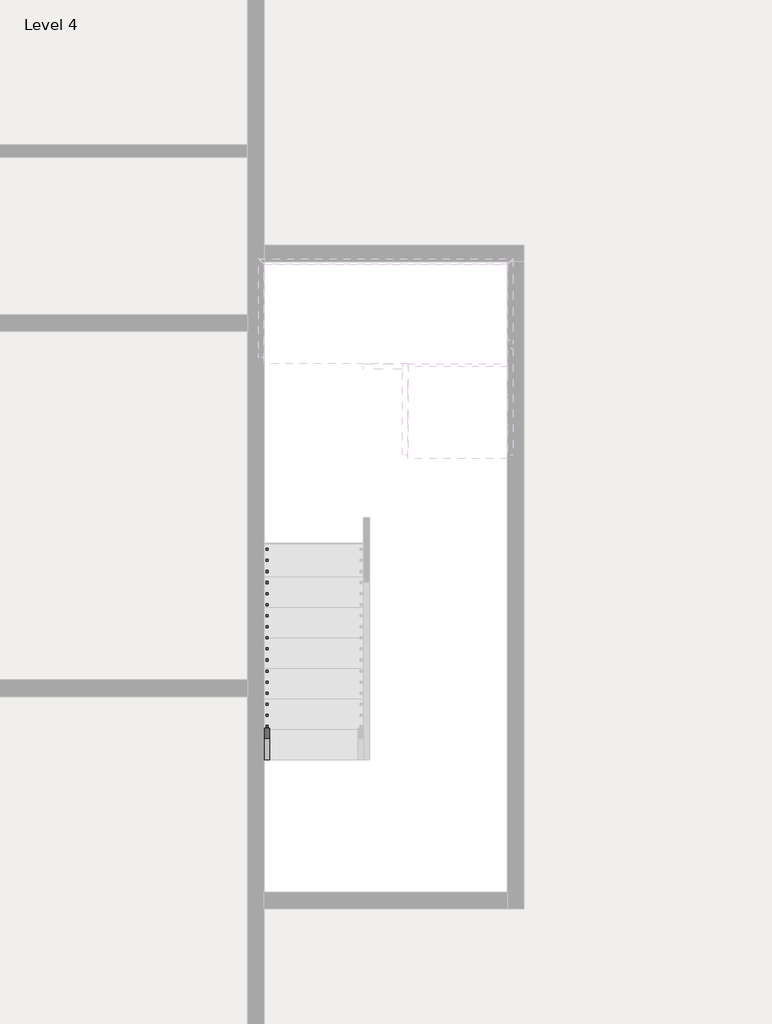
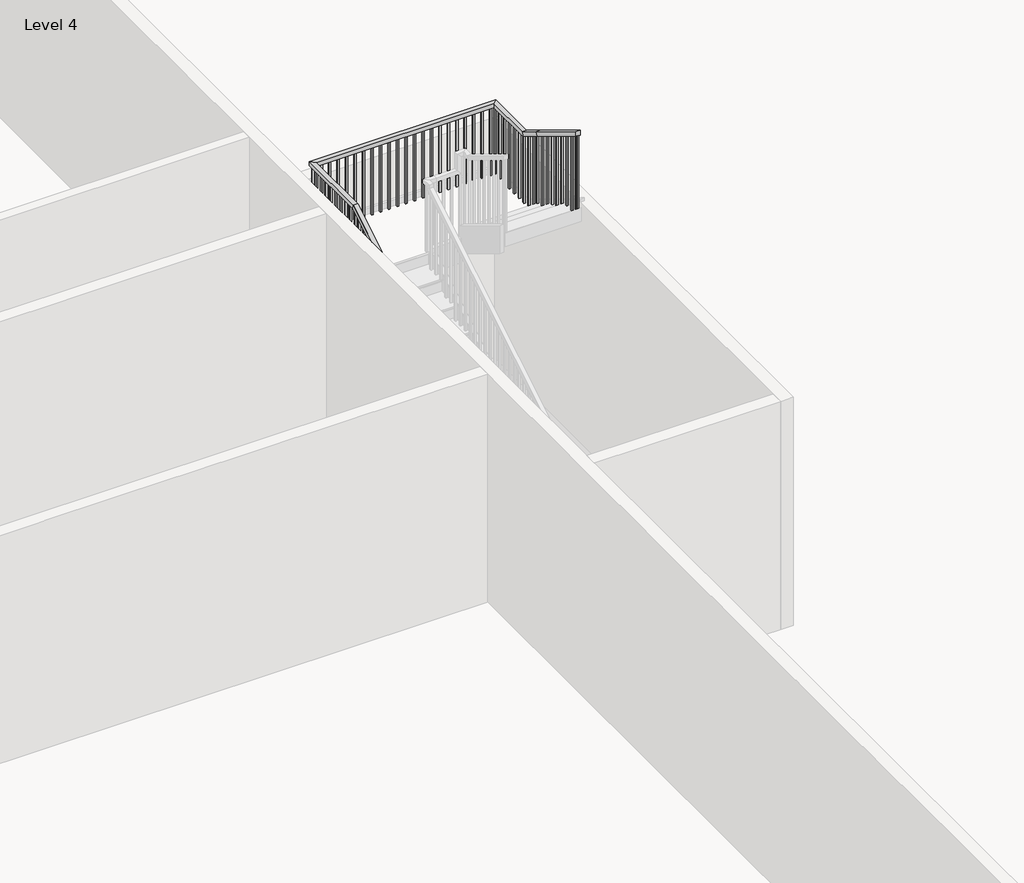
# One storey, part 6 of 8: 1 railing.
"""IFC4 building model written with IfcOpenShell, lengths in millimetres."""

from ifc_helpers import new_model, si_unit, frame, origin, place, context, project, spatial, polyline, outline, extrude, faceted_brep, element, save

model = new_model("IFC4")

# Units and contexts
model_context = context("Model", 3, world=origin())
ifc_project = project(units=[si_unit("LENGTHUNIT", "METRE", prefix="MILLI")], contexts=[model_context])

# Site, building, storey
site = spatial("IfcSite", under=ifc_project)
building = spatial("IfcBuilding", under=site)
storey = spatial("IfcBuildingStorey", under=building, Name="Level 4", Elevation=34378.6172466)

# Railing
placement = place(None, origin())
element("IfcRailing", 1, ObjectType="Handrail - Rectangular", at=placement, inside=storey, context=model_context, shape_type="SolidModel", body=[
    faceted_brep([(-3617.4415084, -23154.3851539, 35462.3505799), (-3617.4415084, -23154.3851539, 35402.9491197), (-3566.6415084, -23154.3851539, 35402.9491197), (-3566.6415084, -23154.3851539, 35462.3505799), (-3617.4415084, -19522.1851539, 37663.6839133), (-3617.4415084, -19507.9927445, 37612.8839133), (-3566.6415084, -19507.9927445, 37612.8839133), (-3566.6415084, -19522.1851539, 37663.6839133), (-3617.4415084, -18607.7851539, 37663.6839133), (-3617.4415084, -18607.7851539, 37612.8839133), (-3566.6415084, -18658.5851539, 37612.8839133), (-3566.6415084, -18658.5851539, 37663.6839133), (-1382.2415084, -18607.7851539, 37663.6839133), (-1382.2415084, -18607.7851539, 37612.8839133), (-1433.0415084, -18658.5851539, 37612.8839133), (-1433.0415084, -18658.5851539, 37663.6839133), (-1382.2415084, -19242.7851539, 37663.6839133), (-1382.2415084, -19256.9775633, 37612.8839133), (-1433.0415084, -19256.9775633, 37612.8839133), (-1433.0415084, -19242.7851539, 37663.6839133), (-1382.2415084, -19522.1851539, 37833.0172466), (-1382.2415084, -19548.5148811, 37789.5731968), (-1433.0415084, -19548.5148811, 37789.5731968), (-1433.0415084, -19522.1851539, 37833.0172466), (-1382.2415084, -20360.3851539, 38341.0172466), (-1433.0415084, -20360.3851539, 38341.0172466), (-1433.0415084, -20360.3851539, 38281.6157863), (-1382.2415084, -20360.3851539, 38281.6157863)], [[[0, 1, 2, 3]], [[1, 0, 4, 5]], [[2, 1, 5, 6]], [[3, 2, 6, 7]], [[0, 3, 7, 4]], [[5, 4, 8, 9]], [[6, 5, 9, 10]], [[7, 6, 10, 11]], [[4, 7, 11, 8]], [[9, 8, 12, 13]], [[10, 9, 13, 14]], [[11, 10, 14, 15]], [[8, 11, 15, 12]], [[13, 12, 16, 17]], [[14, 13, 17, 18]], [[15, 14, 18, 19]], [[12, 15, 19, 16]], [[17, 16, 20, 21]], [[18, 17, 21, 22]], [[19, 18, 22, 23]], [[16, 19, 23, 20]], [[24, 25, 26, 27]], [[21, 20, 24, 27]], [[22, 21, 27, 26]], [[23, 22, 26, 25]], [[20, 23, 25, 24]]]),
    extrude(outline(polyline([(-20325.4601539, 38260.4491197), (-20325.4601539, 37257.2839133), (-20344.5101539, 37257.2839133), (-20344.5101539, 38271.9945742), (-20325.4601539, 38260.4491197)])), frame((-1417.1665084, 0.0, 0.0), z_axis=(1.0, 0.0, 0.0), x_axis=(0.0, 1.0, 0.0)), (0.0, 0.0, 1.0), 19.05),
    extrude(outline(polyline([(-20223.8601539, 38198.8733621), (-20223.8601539, 37257.2839133), (-20242.9101539, 37257.2839133), (-20242.9101539, 38210.4188166), (-20223.8601539, 38198.8733621)])), frame((-1417.1665084, 0.0, 0.0), z_axis=(1.0, 0.0, 0.0), x_axis=(0.0, 1.0, 0.0)), (0.0, 0.0, 1.0), 19.05),
    extrude(outline(polyline([(-20122.2601539, 38137.2976045), (-20122.2601539, 37257.2839133), (-20141.3101539, 37257.2839133), (-20141.3101539, 38148.8430591), (-20122.2601539, 38137.2976045)])), frame((-1417.1665084, 0.0, 0.0), z_axis=(1.0, 0.0, 0.0), x_axis=(0.0, 1.0, 0.0)), (0.0, 0.0, 1.0), 19.05),
    extrude(outline(polyline([(-20020.6601539, 38075.721847), (-20020.6601539, 37087.9505799), (-20039.7101539, 37087.9505799), (-20039.7101539, 38087.2673015), (-20020.6601539, 38075.721847)])), frame((-1417.1665084, 0.0, 0.0), z_axis=(1.0, 0.0, 0.0), x_axis=(0.0, 1.0, 0.0)), (0.0, 0.0, 1.0), 19.05),
    extrude(outline(polyline([(-19919.0601539, 38014.1460894), (-19919.0601539, 37087.9505799), (-19938.1101539, 37087.9505799), (-19938.1101539, 38025.6915439), (-19919.0601539, 38014.1460894)])), frame((-1417.1665084, 0.0, 0.0), z_axis=(1.0, 0.0, 0.0), x_axis=(0.0, 1.0, 0.0)), (0.0, 0.0, 1.0), 19.05),
    extrude(outline(polyline([(-19817.4601539, 37952.5703318), (-19817.4601539, 37087.9505799), (-19836.5101539, 37087.9505799), (-19836.5101539, 37964.1157863), (-19817.4601539, 37952.5703318)])), frame((-1417.1665084, 0.0, 0.0), z_axis=(1.0, 0.0, 0.0), x_axis=(0.0, 1.0, 0.0)), (0.0, 0.0, 1.0), 19.05),
    extrude(outline(polyline([(-19715.8601539, 37890.9945742), (-19715.8601539, 36918.6172466), (-19734.9101539, 36918.6172466), (-19734.9101539, 37902.5400288), (-19715.8601539, 37890.9945742)])), frame((-1417.1665084, 0.0, 0.0), z_axis=(1.0, 0.0, 0.0), x_axis=(0.0, 1.0, 0.0)), (0.0, 0.0, 1.0), 19.05),
    extrude(outline(polyline([(-19614.2601539, 37829.4188166), (-19614.2601539, 36918.6172466), (-19633.3101539, 36918.6172466), (-19633.3101539, 37840.9642712), (-19614.2601539, 37829.4188166)])), frame((-1417.1665084, 0.0, 0.0), z_axis=(1.0, 0.0, 0.0), x_axis=(0.0, 1.0, 0.0)), (0.0, 0.0, 1.0), 19.05),
    extrude(outline(polyline([(-19436.4601539, 37721.6612409), (-19436.4601539, 36749.2839133), (-19455.5101539, 36749.2839133), (-19455.5101539, 37733.2066954), (-19436.4601539, 37721.6612409)])), frame((-1417.1665084, 0.0, 0.0), z_axis=(1.0, 0.0, 0.0), x_axis=(0.0, 1.0, 0.0)), (0.0, 0.0, 1.0), 19.05),
    extrude(outline(polyline([(-19334.8601539, 37660.0854833), (-19334.8601539, 36749.2839133), (-19353.9101539, 36749.2839133), (-19353.9101539, 37671.6309379), (-19334.8601539, 37660.0854833)])), frame((-1417.1665084, 0.0, 0.0), z_axis=(1.0, 0.0, 0.0), x_axis=(0.0, 1.0, 0.0)), (0.0, 0.0, 1.0), 19.05),
    extrude(outline(polyline([(-1398.1165084, -19233.2601539), (-1398.1165084, -19252.3101539), (-1417.1665084, -19252.3101539), (-1417.1665084, -19233.2601539), (-1398.1165084, -19233.2601539)])), frame((0.0, 0.0, 36749.2839133), z_axis=(0.0, 0.0, 1.0), x_axis=(1.0, 0.0, 0.0)), (0.0, 0.0, 1.0), 863.6),
    extrude(outline(polyline([(-1398.1165084, -19131.6601539), (-1398.1165084, -19150.7101539), (-1417.1665084, -19150.7101539), (-1417.1665084, -19131.6601539), (-1398.1165084, -19131.6601539)])), frame((0.0, 0.0, 36749.2839133), z_axis=(0.0, 0.0, 1.0), x_axis=(1.0, 0.0, 0.0)), (0.0, 0.0, 1.0), 863.6),
    extrude(outline(polyline([(-1398.1165084, -19030.0601539), (-1398.1165084, -19049.1101539), (-1417.1665084, -19049.1101539), (-1417.1665084, -19030.0601539), (-1398.1165084, -19030.0601539)])), frame((0.0, 0.0, 36749.2839133), z_axis=(0.0, 0.0, 1.0), x_axis=(1.0, 0.0, 0.0)), (0.0, 0.0, 1.0), 863.6),
    extrude(outline(polyline([(-1398.1165084, -18928.4601539), (-1398.1165084, -18947.5101539), (-1417.1665084, -18947.5101539), (-1417.1665084, -18928.4601539), (-1398.1165084, -18928.4601539)])), frame((0.0, 0.0, 36749.2839133), z_axis=(0.0, 0.0, 1.0), x_axis=(1.0, 0.0, 0.0)), (0.0, 0.0, 1.0), 863.6),
    extrude(outline(polyline([(-1398.1165084, -18826.8601539), (-1398.1165084, -18845.9101539), (-1417.1665084, -18845.9101539), (-1417.1665084, -18826.8601539), (-1398.1165084, -18826.8601539)])), frame((0.0, 0.0, 36749.2839133), z_axis=(0.0, 0.0, 1.0), x_axis=(1.0, 0.0, 0.0)), (0.0, 0.0, 1.0), 863.6),
    extrude(outline(polyline([(-1398.1165084, -18725.2601539), (-1398.1165084, -18744.3101539), (-1417.1665084, -18744.3101539), (-1417.1665084, -18725.2601539), (-1398.1165084, -18725.2601539)])), frame((0.0, 0.0, 36749.2839133), z_axis=(0.0, 0.0, 1.0), x_axis=(1.0, 0.0, 0.0)), (0.0, 0.0, 1.0), 863.6),
    extrude(outline(polyline([(-1467.9665084, -18623.6601539), (-1448.9165084, -18623.6601539), (-1448.9165084, -18642.7101539), (-1467.9665084, -18642.7101539), (-1467.9665084, -18623.6601539)])), frame((0.0, 0.0, 36749.2839133), z_axis=(0.0, 0.0, 1.0), x_axis=(1.0, 0.0, 0.0)), (0.0, 0.0, 1.0), 863.6),
    extrude(outline(polyline([(-1569.5665084, -18623.6601539), (-1550.5165084, -18623.6601539), (-1550.5165084, -18642.7101539), (-1569.5665084, -18642.7101539), (-1569.5665084, -18623.6601539)])), frame((0.0, 0.0, 36749.2839133), z_axis=(0.0, 0.0, 1.0), x_axis=(1.0, 0.0, 0.0)), (0.0, 0.0, 1.0), 863.6),
    extrude(outline(polyline([(-1671.1665084, -18623.6601539), (-1652.1165084, -18623.6601539), (-1652.1165084, -18642.7101539), (-1671.1665084, -18642.7101539), (-1671.1665084, -18623.6601539)])), frame((0.0, 0.0, 36749.2839133), z_axis=(0.0, 0.0, 1.0), x_axis=(1.0, 0.0, 0.0)), (0.0, 0.0, 1.0), 863.6),
    extrude(outline(polyline([(-1772.7665084, -18623.6601539), (-1753.7165084, -18623.6601539), (-1753.7165084, -18642.7101539), (-1772.7665084, -18642.7101539), (-1772.7665084, -18623.6601539)])), frame((0.0, 0.0, 36749.2839133), z_axis=(0.0, 0.0, 1.0), x_axis=(1.0, 0.0, 0.0)), (0.0, 0.0, 1.0), 863.6),
    extrude(outline(polyline([(-1874.3665084, -18623.6601539), (-1855.3165084, -18623.6601539), (-1855.3165084, -18642.7101539), (-1874.3665084, -18642.7101539), (-1874.3665084, -18623.6601539)])), frame((0.0, 0.0, 36749.2839133), z_axis=(0.0, 0.0, 1.0), x_axis=(1.0, 0.0, 0.0)), (0.0, 0.0, 1.0), 863.6),
    extrude(outline(polyline([(-1975.9665084, -18623.6601539), (-1956.9165084, -18623.6601539), (-1956.9165084, -18642.7101539), (-1975.9665084, -18642.7101539), (-1975.9665084, -18623.6601539)])), frame((0.0, 0.0, 36749.2839133), z_axis=(0.0, 0.0, 1.0), x_axis=(1.0, 0.0, 0.0)), (0.0, 0.0, 1.0), 863.6),
    extrude(outline(polyline([(-2077.5665084, -18623.6601539), (-2058.5165084, -18623.6601539), (-2058.5165084, -18642.7101539), (-2077.5665084, -18642.7101539), (-2077.5665084, -18623.6601539)])), frame((0.0, 0.0, 36749.2839133), z_axis=(0.0, 0.0, 1.0), x_axis=(1.0, 0.0, 0.0)), (0.0, 0.0, 1.0), 863.6),
    extrude(outline(polyline([(-2179.1665084, -18623.6601539), (-2160.1165084, -18623.6601539), (-2160.1165084, -18642.7101539), (-2179.1665084, -18642.7101539), (-2179.1665084, -18623.6601539)])), frame((0.0, 0.0, 36749.2839133), z_axis=(0.0, 0.0, 1.0), x_axis=(1.0, 0.0, 0.0)), (0.0, 0.0, 1.0), 863.6),
    extrude(outline(polyline([(-2280.7665084, -18623.6601539), (-2261.7165084, -18623.6601539), (-2261.7165084, -18642.7101539), (-2280.7665084, -18642.7101539), (-2280.7665084, -18623.6601539)])), frame((0.0, 0.0, 36749.2839133), z_axis=(0.0, 0.0, 1.0), x_axis=(1.0, 0.0, 0.0)), (0.0, 0.0, 1.0), 863.6),
    extrude(outline(polyline([(-2382.3665084, -18623.6601539), (-2363.3165084, -18623.6601539), (-2363.3165084, -18642.7101539), (-2382.3665084, -18642.7101539), (-2382.3665084, -18623.6601539)])), frame((0.0, 0.0, 36749.2839133), z_axis=(0.0, 0.0, 1.0), x_axis=(1.0, 0.0, 0.0)), (0.0, 0.0, 1.0), 863.6),
    extrude(outline(polyline([(-2483.9665084, -18623.6601539), (-2464.9165084, -18623.6601539), (-2464.9165084, -18642.7101539), (-2483.9665084, -18642.7101539), (-2483.9665084, -18623.6601539)])), frame((0.0, 0.0, 36749.2839133), z_axis=(0.0, 0.0, 1.0), x_axis=(1.0, 0.0, 0.0)), (0.0, 0.0, 1.0), 863.6),
    extrude(outline(polyline([(-2585.5665084, -18623.6601539), (-2566.5165084, -18623.6601539), (-2566.5165084, -18642.7101539), (-2585.5665084, -18642.7101539), (-2585.5665084, -18623.6601539)])), frame((0.0, 0.0, 36749.2839133), z_axis=(0.0, 0.0, 1.0), x_axis=(1.0, 0.0, 0.0)), (0.0, 0.0, 1.0), 863.6),
    extrude(outline(polyline([(-2687.1665084, -18623.6601539), (-2668.1165084, -18623.6601539), (-2668.1165084, -18642.7101539), (-2687.1665084, -18642.7101539), (-2687.1665084, -18623.6601539)])), frame((0.0, 0.0, 36749.2839133), z_axis=(0.0, 0.0, 1.0), x_axis=(1.0, 0.0, 0.0)), (0.0, 0.0, 1.0), 863.6),
    extrude(outline(polyline([(-2788.7665084, -18623.6601539), (-2769.7165084, -18623.6601539), (-2769.7165084, -18642.7101539), (-2788.7665084, -18642.7101539), (-2788.7665084, -18623.6601539)])), frame((0.0, 0.0, 36749.2839133), z_axis=(0.0, 0.0, 1.0), x_axis=(1.0, 0.0, 0.0)), (0.0, 0.0, 1.0), 863.6),
    extrude(outline(polyline([(-2890.3665084, -18623.6601539), (-2871.3165084, -18623.6601539), (-2871.3165084, -18642.7101539), (-2890.3665084, -18642.7101539), (-2890.3665084, -18623.6601539)])), frame((0.0, 0.0, 36749.2839133), z_axis=(0.0, 0.0, 1.0), x_axis=(1.0, 0.0, 0.0)), (0.0, 0.0, 1.0), 863.6),
    extrude(outline(polyline([(-2991.9665084, -18623.6601539), (-2972.9165084, -18623.6601539), (-2972.9165084, -18642.7101539), (-2991.9665084, -18642.7101539), (-2991.9665084, -18623.6601539)])), frame((0.0, 0.0, 36749.2839133), z_axis=(0.0, 0.0, 1.0), x_axis=(1.0, 0.0, 0.0)), (0.0, 0.0, 1.0), 863.6),
    extrude(outline(polyline([(-3093.5665084, -18623.6601539), (-3074.5165084, -18623.6601539), (-3074.5165084, -18642.7101539), (-3093.5665084, -18642.7101539), (-3093.5665084, -18623.6601539)])), frame((0.0, 0.0, 36749.2839133), z_axis=(0.0, 0.0, 1.0), x_axis=(1.0, 0.0, 0.0)), (0.0, 0.0, 1.0), 863.6),
    extrude(outline(polyline([(-3195.1665084, -18623.6601539), (-3176.1165084, -18623.6601539), (-3176.1165084, -18642.7101539), (-3195.1665084, -18642.7101539), (-3195.1665084, -18623.6601539)])), frame((0.0, 0.0, 36749.2839133), z_axis=(0.0, 0.0, 1.0), x_axis=(1.0, 0.0, 0.0)), (0.0, 0.0, 1.0), 863.6),
    extrude(outline(polyline([(-3296.7665084, -18623.6601539), (-3277.7165084, -18623.6601539), (-3277.7165084, -18642.7101539), (-3296.7665084, -18642.7101539), (-3296.7665084, -18623.6601539)])), frame((0.0, 0.0, 36749.2839133), z_axis=(0.0, 0.0, 1.0), x_axis=(1.0, 0.0, 0.0)), (0.0, 0.0, 1.0), 863.6),
    extrude(outline(polyline([(-3398.3665084, -18623.6601539), (-3379.3165084, -18623.6601539), (-3379.3165084, -18642.7101539), (-3398.3665084, -18642.7101539), (-3398.3665084, -18623.6601539)])), frame((0.0, 0.0, 36749.2839133), z_axis=(0.0, 0.0, 1.0), x_axis=(1.0, 0.0, 0.0)), (0.0, 0.0, 1.0), 863.6),
    extrude(outline(polyline([(-3499.9665084, -18623.6601539), (-3480.9165084, -18623.6601539), (-3480.9165084, -18642.7101539), (-3499.9665084, -18642.7101539), (-3499.9665084, -18623.6601539)])), frame((0.0, 0.0, 36749.2839133), z_axis=(0.0, 0.0, 1.0), x_axis=(1.0, 0.0, 0.0)), (0.0, 0.0, 1.0), 863.6),
    extrude(outline(polyline([(-3601.5665084, -18718.9101539), (-3601.5665084, -18699.8601539), (-3582.5165084, -18699.8601539), (-3582.5165084, -18718.9101539), (-3601.5665084, -18718.9101539)])), frame((0.0, 0.0, 36749.2839133), z_axis=(0.0, 0.0, 1.0), x_axis=(1.0, 0.0, 0.0)), (0.0, 0.0, 1.0), 863.6),
    extrude(outline(polyline([(-3601.5665084, -18820.5101539), (-3601.5665084, -18801.4601539), (-3582.5165084, -18801.4601539), (-3582.5165084, -18820.5101539), (-3601.5665084, -18820.5101539)])), frame((0.0, 0.0, 36749.2839133), z_axis=(0.0, 0.0, 1.0), x_axis=(1.0, 0.0, 0.0)), (0.0, 0.0, 1.0), 863.6),
    extrude(outline(polyline([(-3601.5665084, -18922.1101539), (-3601.5665084, -18903.0601539), (-3582.5165084, -18903.0601539), (-3582.5165084, -18922.1101539), (-3601.5665084, -18922.1101539)])), frame((0.0, 0.0, 36749.2839133), z_axis=(0.0, 0.0, 1.0), x_axis=(1.0, 0.0, 0.0)), (0.0, 0.0, 1.0), 863.6),
    extrude(outline(polyline([(-3601.5665084, -19023.7101539), (-3601.5665084, -19004.6601539), (-3582.5165084, -19004.6601539), (-3582.5165084, -19023.7101539), (-3601.5665084, -19023.7101539)])), frame((0.0, 0.0, 36749.2839133), z_axis=(0.0, 0.0, 1.0), x_axis=(1.0, 0.0, 0.0)), (0.0, 0.0, 1.0), 863.6),
    extrude(outline(polyline([(-3601.5665084, -19125.3101539), (-3601.5665084, -19106.2601539), (-3582.5165084, -19106.2601539), (-3582.5165084, -19125.3101539), (-3601.5665084, -19125.3101539)])), frame((0.0, 0.0, 36749.2839133), z_axis=(0.0, 0.0, 1.0), x_axis=(1.0, 0.0, 0.0)), (0.0, 0.0, 1.0), 863.6),
    extrude(outline(polyline([(-3601.5665084, -19226.9101539), (-3601.5665084, -19207.8601539), (-3582.5165084, -19207.8601539), (-3582.5165084, -19226.9101539), (-3601.5665084, -19226.9101539)])), frame((0.0, 0.0, 36749.2839133), z_axis=(0.0, 0.0, 1.0), x_axis=(1.0, 0.0, 0.0)), (0.0, 0.0, 1.0), 863.6),
    extrude(outline(polyline([(-3601.5665084, -19328.5101539), (-3601.5665084, -19309.4601539), (-3582.5165084, -19309.4601539), (-3582.5165084, -19328.5101539), (-3601.5665084, -19328.5101539)])), frame((0.0, 0.0, 36749.2839133), z_axis=(0.0, 0.0, 1.0), x_axis=(1.0, 0.0, 0.0)), (0.0, 0.0, 1.0), 863.6),
    extrude(outline(polyline([(-3601.5665084, -19430.1101539), (-3601.5665084, -19411.0601539), (-3582.5165084, -19411.0601539), (-3582.5165084, -19430.1101539), (-3601.5665084, -19430.1101539)])), frame((0.0, 0.0, 36749.2839133), z_axis=(0.0, 0.0, 1.0), x_axis=(1.0, 0.0, 0.0)), (0.0, 0.0, 1.0), 863.6),
    extrude(outline(polyline([(-19588.8601539, 37563.8733621), (-19588.8601539, 36579.9505799), (-19607.9101539, 36579.9505799), (-19607.9101539, 37552.3279076), (-19588.8601539, 37563.8733621)])), frame((-3601.5665084, 0.0, 0.0), z_axis=(1.0, 0.0, 0.0), x_axis=(0.0, 1.0, 0.0)), (0.0, 0.0, 1.0), 19.05),
    extrude(outline(polyline([(-19690.4601539, 37502.2976045), (-19690.4601539, 36579.9505799), (-19709.5101539, 36579.9505799), (-19709.5101539, 37490.75215), (-19690.4601539, 37502.2976045)])), frame((-3601.5665084, 0.0, 0.0), z_axis=(1.0, 0.0, 0.0), x_axis=(0.0, 1.0, 0.0)), (0.0, 0.0, 1.0), 19.05),
    extrude(outline(polyline([(-19792.0601539, 37440.721847), (-19792.0601539, 36579.9505799), (-19811.1101539, 36579.9505799), (-19811.1101539, 37429.1763924), (-19792.0601539, 37440.721847)])), frame((-3601.5665084, 0.0, 0.0), z_axis=(1.0, 0.0, 0.0), x_axis=(0.0, 1.0, 0.0)), (0.0, 0.0, 1.0), 19.05),
    extrude(outline(polyline([(-19893.6601539, 37379.1460894), (-19893.6601539, 36410.6172466), (-19912.7101539, 36410.6172466), (-19912.7101539, 37367.6006348), (-19893.6601539, 37379.1460894)])), frame((-3601.5665084, 0.0, 0.0), z_axis=(1.0, 0.0, 0.0), x_axis=(0.0, 1.0, 0.0)), (0.0, 0.0, 1.0), 19.05),
    extrude(outline(polyline([(-19995.2601539, 37317.5703318), (-19995.2601539, 36410.6172466), (-20014.3101539, 36410.6172466), (-20014.3101539, 37306.0248773), (-19995.2601539, 37317.5703318)])), frame((-3601.5665084, 0.0, 0.0), z_axis=(1.0, 0.0, 0.0), x_axis=(0.0, 1.0, 0.0)), (0.0, 0.0, 1.0), 19.05),
    extrude(outline(polyline([(-20096.8601539, 37255.9945742), (-20096.8601539, 36241.2839133), (-20115.9101539, 36241.2839133), (-20115.9101539, 37244.4491197), (-20096.8601539, 37255.9945742)])), frame((-3601.5665084, 0.0, 0.0), z_axis=(1.0, 0.0, 0.0), x_axis=(0.0, 1.0, 0.0)), (0.0, 0.0, 1.0), 19.05),
    extrude(outline(polyline([(-20198.4601539, 37194.4188166), (-20198.4601539, 36241.2839133), (-20217.5101539, 36241.2839133), (-20217.5101539, 37182.8733621), (-20198.4601539, 37194.4188166)])), frame((-3601.5665084, 0.0, 0.0), z_axis=(1.0, 0.0, 0.0), x_axis=(0.0, 1.0, 0.0)), (0.0, 0.0, 1.0), 19.05),
    extrude(outline(polyline([(-20300.0601539, 37132.8430591), (-20300.0601539, 36241.2839133), (-20319.1101539, 36241.2839133), (-20319.1101539, 37121.2976045), (-20300.0601539, 37132.8430591)])), frame((-3601.5665084, 0.0, 0.0), z_axis=(1.0, 0.0, 0.0), x_axis=(0.0, 1.0, 0.0)), (0.0, 0.0, 1.0), 19.05),
    extrude(outline(polyline([(-20401.6601539, 37071.2673015), (-20401.6601539, 36071.9505799), (-20420.7101539, 36071.9505799), (-20420.7101539, 37059.721847), (-20401.6601539, 37071.2673015)])), frame((-3601.5665084, 0.0, 0.0), z_axis=(1.0, 0.0, 0.0), x_axis=(0.0, 1.0, 0.0)), (0.0, 0.0, 1.0), 19.05),
    extrude(outline(polyline([(-20503.2601539, 37009.6915439), (-20503.2601539, 36071.9505799), (-20522.3101539, 36071.9505799), (-20522.3101539, 36998.1460894), (-20503.2601539, 37009.6915439)])), frame((-3601.5665084, 0.0, 0.0), z_axis=(1.0, 0.0, 0.0), x_axis=(0.0, 1.0, 0.0)), (0.0, 0.0, 1.0), 19.05),
    extrude(outline(polyline([(-20604.8601539, 36948.1157863), (-20604.8601539, 36071.9505799), (-20623.9101539, 36071.9505799), (-20623.9101539, 36936.5703318), (-20604.8601539, 36948.1157863)])), frame((-3601.5665084, 0.0, 0.0), z_axis=(1.0, 0.0, 0.0), x_axis=(0.0, 1.0, 0.0)), (0.0, 0.0, 1.0), 19.05),
    extrude(outline(polyline([(-20706.4601539, 36886.5400288), (-20706.4601539, 35902.6172466), (-20725.5101539, 35902.6172466), (-20725.5101539, 36874.9945742), (-20706.4601539, 36886.5400288)])), frame((-3601.5665084, 0.0, 0.0), z_axis=(1.0, 0.0, 0.0), x_axis=(0.0, 1.0, 0.0)), (0.0, 0.0, 1.0), 19.05),
    extrude(outline(polyline([(-20808.0601539, 36824.9642712), (-20808.0601539, 35902.6172466), (-20827.1101539, 35902.6172466), (-20827.1101539, 36813.4188166), (-20808.0601539, 36824.9642712)])), frame((-3601.5665084, 0.0, 0.0), z_axis=(1.0, 0.0, 0.0), x_axis=(0.0, 1.0, 0.0)), (0.0, 0.0, 1.0), 19.05),
    extrude(outline(polyline([(-20909.6601539, 36763.3885136), (-20909.6601539, 35902.6172466), (-20928.7101539, 35902.6172466), (-20928.7101539, 36751.8430591), (-20909.6601539, 36763.3885136)])), frame((-3601.5665084, 0.0, 0.0), z_axis=(1.0, 0.0, 0.0), x_axis=(0.0, 1.0, 0.0)), (0.0, 0.0, 1.0), 19.05),
    extrude(outline(polyline([(-21011.2601539, 36701.812756), (-21011.2601539, 35733.2839133), (-21030.3101539, 35733.2839133), (-21030.3101539, 36690.2673015), (-21011.2601539, 36701.812756)])), frame((-3601.5665084, 0.0, 0.0), z_axis=(1.0, 0.0, 0.0), x_axis=(0.0, 1.0, 0.0)), (0.0, 0.0, 1.0), 19.05),
    extrude(outline(polyline([(-21112.8601539, 36640.2369985), (-21112.8601539, 35733.2839133), (-21131.9101539, 35733.2839133), (-21131.9101539, 36628.6915439), (-21112.8601539, 36640.2369985)])), frame((-3601.5665084, 0.0, 0.0), z_axis=(1.0, 0.0, 0.0), x_axis=(0.0, 1.0, 0.0)), (0.0, 0.0, 1.0), 19.05),
    extrude(outline(polyline([(-21214.4601539, 36578.6612409), (-21214.4601539, 35563.9505799), (-21233.5101539, 35563.9505799), (-21233.5101539, 36567.1157863), (-21214.4601539, 36578.6612409)])), frame((-3601.5665084, 0.0, 0.0), z_axis=(1.0, 0.0, 0.0), x_axis=(0.0, 1.0, 0.0)), (0.0, 0.0, 1.0), 19.05),
    extrude(outline(polyline([(-21316.0601539, 36517.0854833), (-21316.0601539, 35563.9505799), (-21335.1101539, 35563.9505799), (-21335.1101539, 36505.5400288), (-21316.0601539, 36517.0854833)])), frame((-3601.5665084, 0.0, 0.0), z_axis=(1.0, 0.0, 0.0), x_axis=(0.0, 1.0, 0.0)), (0.0, 0.0, 1.0), 19.05),
    extrude(outline(polyline([(-21417.6601539, 36455.5097257), (-21417.6601539, 35563.9505799), (-21436.7101539, 35563.9505799), (-21436.7101539, 36443.9642712), (-21417.6601539, 36455.5097257)])), frame((-3601.5665084, 0.0, 0.0), z_axis=(1.0, 0.0, 0.0), x_axis=(0.0, 1.0, 0.0)), (0.0, 0.0, 1.0), 19.05),
    extrude(outline(polyline([(-21519.2601539, 36393.9339682), (-21519.2601539, 35394.6172466), (-21538.3101539, 35394.6172466), (-21538.3101539, 36382.3885136), (-21519.2601539, 36393.9339682)])), frame((-3601.5665084, 0.0, 0.0), z_axis=(1.0, 0.0, 0.0), x_axis=(0.0, 1.0, 0.0)), (0.0, 0.0, 1.0), 19.05),
    extrude(outline(polyline([(-21620.8601539, 36332.3582106), (-21620.8601539, 35394.6172466), (-21639.9101539, 35394.6172466), (-21639.9101539, 36320.812756), (-21620.8601539, 36332.3582106)])), frame((-3601.5665084, 0.0, 0.0), z_axis=(1.0, 0.0, 0.0), x_axis=(0.0, 1.0, 0.0)), (0.0, 0.0, 1.0), 19.05),
    extrude(outline(polyline([(-21722.4601539, 36270.782453), (-21722.4601539, 35394.6172466), (-21741.5101539, 35394.6172466), (-21741.5101539, 36259.2369985), (-21722.4601539, 36270.782453)])), frame((-3601.5665084, 0.0, 0.0), z_axis=(1.0, 0.0, 0.0), x_axis=(0.0, 1.0, 0.0)), (0.0, 0.0, 1.0), 19.05),
    extrude(outline(polyline([(-21824.0601539, 36209.2066954), (-21824.0601539, 35225.2839133), (-21843.1101539, 35225.2839133), (-21843.1101539, 36197.6612409), (-21824.0601539, 36209.2066954)])), frame((-3601.5665084, 0.0, 0.0), z_axis=(1.0, 0.0, 0.0), x_axis=(0.0, 1.0, 0.0)), (0.0, 0.0, 1.0), 19.05),
    extrude(outline(polyline([(-21925.6601539, 36147.6309379), (-21925.6601539, 35225.2839133), (-21944.7101539, 35225.2839133), (-21944.7101539, 36136.0854833), (-21925.6601539, 36147.6309379)])), frame((-3601.5665084, 0.0, 0.0), z_axis=(1.0, 0.0, 0.0), x_axis=(0.0, 1.0, 0.0)), (0.0, 0.0, 1.0), 19.05),
    extrude(outline(polyline([(-22027.2601539, 36086.0551803), (-22027.2601539, 35225.2839133), (-22046.3101539, 35225.2839133), (-22046.3101539, 36074.5097257), (-22027.2601539, 36086.0551803)])), frame((-3601.5665084, 0.0, 0.0), z_axis=(1.0, 0.0, 0.0), x_axis=(0.0, 1.0, 0.0)), (0.0, 0.0, 1.0), 19.05),
    extrude(outline(polyline([(-22128.8601539, 36024.4794227), (-22128.8601539, 35055.9505799), (-22147.9101539, 35055.9505799), (-22147.9101539, 36012.9339682), (-22128.8601539, 36024.4794227)])), frame((-3601.5665084, 0.0, 0.0), z_axis=(1.0, 0.0, 0.0), x_axis=(0.0, 1.0, 0.0)), (0.0, 0.0, 1.0), 19.05),
    extrude(outline(polyline([(-22230.4601539, 35962.9036651), (-22230.4601539, 35055.9505799), (-22249.5101539, 35055.9505799), (-22249.5101539, 35951.3582106), (-22230.4601539, 35962.9036651)])), frame((-3601.5665084, 0.0, 0.0), z_axis=(1.0, 0.0, 0.0), x_axis=(0.0, 1.0, 0.0)), (0.0, 0.0, 1.0), 19.05),
    extrude(outline(polyline([(-22332.0601539, 35901.3279076), (-22332.0601539, 34886.6172466), (-22351.1101539, 34886.6172466), (-22351.1101539, 35889.782453), (-22332.0601539, 35901.3279076)])), frame((-3601.5665084, 0.0, 0.0), z_axis=(1.0, 0.0, 0.0), x_axis=(0.0, 1.0, 0.0)), (0.0, 0.0, 1.0), 19.05),
    extrude(outline(polyline([(-22433.6601539, 35839.75215), (-22433.6601539, 34886.6172466), (-22452.7101539, 34886.6172466), (-22452.7101539, 35828.2066954), (-22433.6601539, 35839.75215)])), frame((-3601.5665084, 0.0, 0.0), z_axis=(1.0, 0.0, 0.0), x_axis=(0.0, 1.0, 0.0)), (0.0, 0.0, 1.0), 19.05),
    extrude(outline(polyline([(-22535.2601539, 35778.1763924), (-22535.2601539, 34886.6172466), (-22554.3101539, 34886.6172466), (-22554.3101539, 35766.6309379), (-22535.2601539, 35778.1763924)])), frame((-3601.5665084, 0.0, 0.0), z_axis=(1.0, 0.0, 0.0), x_axis=(0.0, 1.0, 0.0)), (0.0, 0.0, 1.0), 19.05),
    extrude(outline(polyline([(-22636.8601539, 35716.6006348), (-22636.8601539, 34717.2839133), (-22655.9101539, 34717.2839133), (-22655.9101539, 35705.0551803), (-22636.8601539, 35716.6006348)])), frame((-3601.5665084, 0.0, 0.0), z_axis=(1.0, 0.0, 0.0), x_axis=(0.0, 1.0, 0.0)), (0.0, 0.0, 1.0), 19.05),
    extrude(outline(polyline([(-22738.4601539, 35655.0248773), (-22738.4601539, 34717.2839133), (-22757.5101539, 34717.2839133), (-22757.5101539, 35643.4794227), (-22738.4601539, 35655.0248773)])), frame((-3601.5665084, 0.0, 0.0), z_axis=(1.0, 0.0, 0.0), x_axis=(0.0, 1.0, 0.0)), (0.0, 0.0, 1.0), 19.05),
    extrude(outline(polyline([(-22840.0601539, 35593.4491197), (-22840.0601539, 34717.2839133), (-22859.1101539, 34717.2839133), (-22859.1101539, 35581.9036651), (-22840.0601539, 35593.4491197)])), frame((-3601.5665084, 0.0, 0.0), z_axis=(1.0, 0.0, 0.0), x_axis=(0.0, 1.0, 0.0)), (0.0, 0.0, 1.0), 19.05),
    extrude(outline(polyline([(-22941.6601539, 35531.8733621), (-22941.6601539, 34547.9505799), (-22960.7101539, 34547.9505799), (-22960.7101539, 35520.3279076), (-22941.6601539, 35531.8733621)])), frame((-3601.5665084, 0.0, 0.0), z_axis=(1.0, 0.0, 0.0), x_axis=(0.0, 1.0, 0.0)), (0.0, 0.0, 1.0), 19.05),
    extrude(outline(polyline([(-23043.2601539, 35470.2976045), (-23043.2601539, 34547.9505799), (-23062.3101539, 34547.9505799), (-23062.3101539, 35458.75215), (-23043.2601539, 35470.2976045)])), frame((-3601.5665084, 0.0, 0.0), z_axis=(1.0, 0.0, 0.0), x_axis=(0.0, 1.0, 0.0)), (0.0, 0.0, 1.0), 19.05),
    extrude(outline(polyline([(-19512.6601539, 37767.8430591), (-19512.6601539, 36749.2839133), (-19531.7101539, 36749.2839133), (-19531.7101539, 37779.3885136), (-19512.6601539, 37767.8430591)])), frame((-1417.1665084, 0.0, 0.0), z_axis=(1.0, 0.0, 0.0), x_axis=(0.0, 1.0, 0.0)), (0.0, 0.0, 1.0), 19.05),
    extrude(outline(polyline([(-1417.1665084, -18623.6601539), (-1398.1165084, -18623.6601539), (-1398.1165084, -18642.7101539), (-1417.1665084, -18642.7101539), (-1417.1665084, -18623.6601539)])), frame((0.0, 0.0, 36749.2839133), z_axis=(0.0, 0.0, 1.0), x_axis=(1.0, 0.0, 0.0)), (0.0, 0.0, 1.0), 863.6),
    extrude(outline(polyline([(-3601.5665084, -18642.7101539), (-3601.5665084, -18623.6601539), (-3582.5165084, -18623.6601539), (-3582.5165084, -18642.7101539), (-3601.5665084, -18642.7101539)])), frame((0.0, 0.0, 36749.2839133), z_axis=(0.0, 0.0, 1.0), x_axis=(1.0, 0.0, 0.0)), (0.0, 0.0, 1.0), 863.6),
    extrude(outline(polyline([(-19512.6601539, 37610.0551803), (-19512.6601539, 36749.2839133), (-19531.7101539, 36749.2839133), (-19531.7101539, 37598.5097257), (-19512.6601539, 37610.0551803)])), frame((-3601.5665084, 0.0, 0.0), z_axis=(1.0, 0.0, 0.0), x_axis=(0.0, 1.0, 0.0)), (0.0, 0.0, 1.0), 19.05),
    extrude(outline(polyline([(-20341.3351539, 38270.0703318), (-20341.3351539, 37257.2839133), (-20360.3851539, 37257.2839133), (-20360.3851539, 38281.6157863), (-20341.3351539, 38270.0703318)])), frame((-1417.1665084, 0.0, 0.0), z_axis=(1.0, 0.0, 0.0), x_axis=(0.0, 1.0, 0.0)), (0.0, 0.0, 1.0), 19.05),
    extrude(outline(polyline([(-23135.3351539, 35414.4945742), (-23135.3351539, 34547.9505799), (-23154.3851539, 34547.9505799), (-23154.3851539, 35402.9491197), (-23135.3351539, 35414.4945742)])), frame((-3601.5665084, 0.0, 0.0), z_axis=(1.0, 0.0, 0.0), x_axis=(0.0, 1.0, 0.0)), (0.0, 0.0, 1.0), 19.05),
])

save(model, "model.ifc")

# Revit data of these elements
# Type "Handrail - Rectangular"
#   Assembly Code = "C2010400"
#   built-in parameter 1008612 = 0.0416667 (stored number, unit not read)
#   built-in parameter 1008611 = 0.0416667 (stored number, unit not read)
#   built-in parameter 1008609 = 0.333333 (stored number, unit not read)
#   built-in parameter 1008604 = 0.166667 (stored number, unit not read)
#   built-in parameter 1008603 = 0.166667 (stored number, unit not read)
#   Railing Height = 3' - 0"
#   built-in parameter 1008630 = 2
#   built-in parameter 1008610 = 2
#   built-in parameter 1008618 = Baluster - Square : 3/4"
# Element 1 (IfcRailing, "Handrail - Rectangular")
#   Phase Created = New Construction
